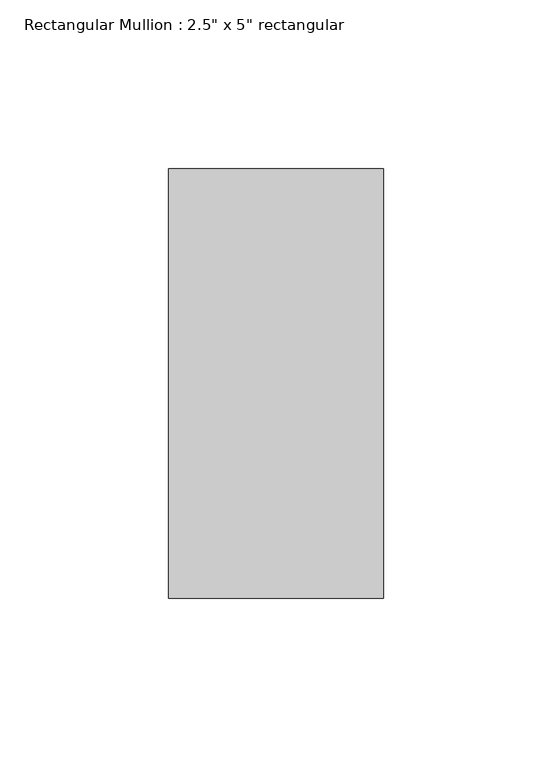
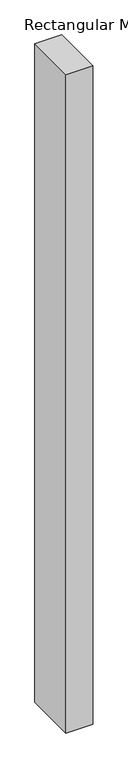
"""IFC4 building model written with IfcOpenShell, lengths in millimetres: member geometry."""

from ifc_helpers import new_model, si_unit, frame, origin, place, context, project, spatial, polyline, outline, extrude, source, transform, mapped, element, save


def member_e2451291(model_context):
    return source(origin(), model_context, "Body", "SweptSolid", [
        extrude(outline(polyline([(31.75, 63.5), (31.75, -63.5), (-31.75, -63.5), (-31.75, 63.5), (31.75, 63.5)])), frame((0.0, 0.0, -1645.4701172), z_axis=(0.0, 0.0, 1.0), x_axis=(1.0, 0.0, 0.0)), (0.0, 0.0, 1.0), 1645.4701172),
    ])


if __name__ == "__main__":
    model = new_model("IFC4")
    model_context = context("Model", 3, world=origin())
    ifc_project = project(units=[si_unit("LENGTHUNIT", "METRE", prefix="MILLI")], contexts=[model_context])
    site = spatial("IfcSite", under=ifc_project)
    building = spatial("IfcBuilding", under=site)
    placement = place(None, origin())
    member_shape = member_e2451291(model_context)
    element("IfcMember", 1, ObjectType="Rectangular Mullion : 2.5\" x 5\" rectangular", at=placement, inside=building, context=model_context, shape_type="MappedRepresentation", body=[
        mapped(member_shape, transform((0.0, 0.0, 0.0), x_axis=(1.0, 0.0, 0.0), y_axis=(0.0, 1.0, 0.0), z_axis=(0.0, 0.0, 1.0))),
    ])
    save(model, "model.ifc")

# Revit data of these elements
# Type "Rectangular Mullion : 2.5\" x 5\" rectangular"
#   built-in parameter 1007304 = 0.416667 (stored number, unit not read)
#   built-in parameter 1007301 = 0.104167 (stored number, unit not read)
#   built-in parameter 1007300 = 0.104167 (stored number, unit not read)
# Element 1 (IfcMember, "Rectangular Mullion : 2.5\" x 5\" rectangular")
#   Materials on its faces: "Aluminum"
# Materials
#   "Aluminum": class "Metal", colour RGB 247 247 247, transparency 0, Description = "Aluminum 6061", Cost = 0
